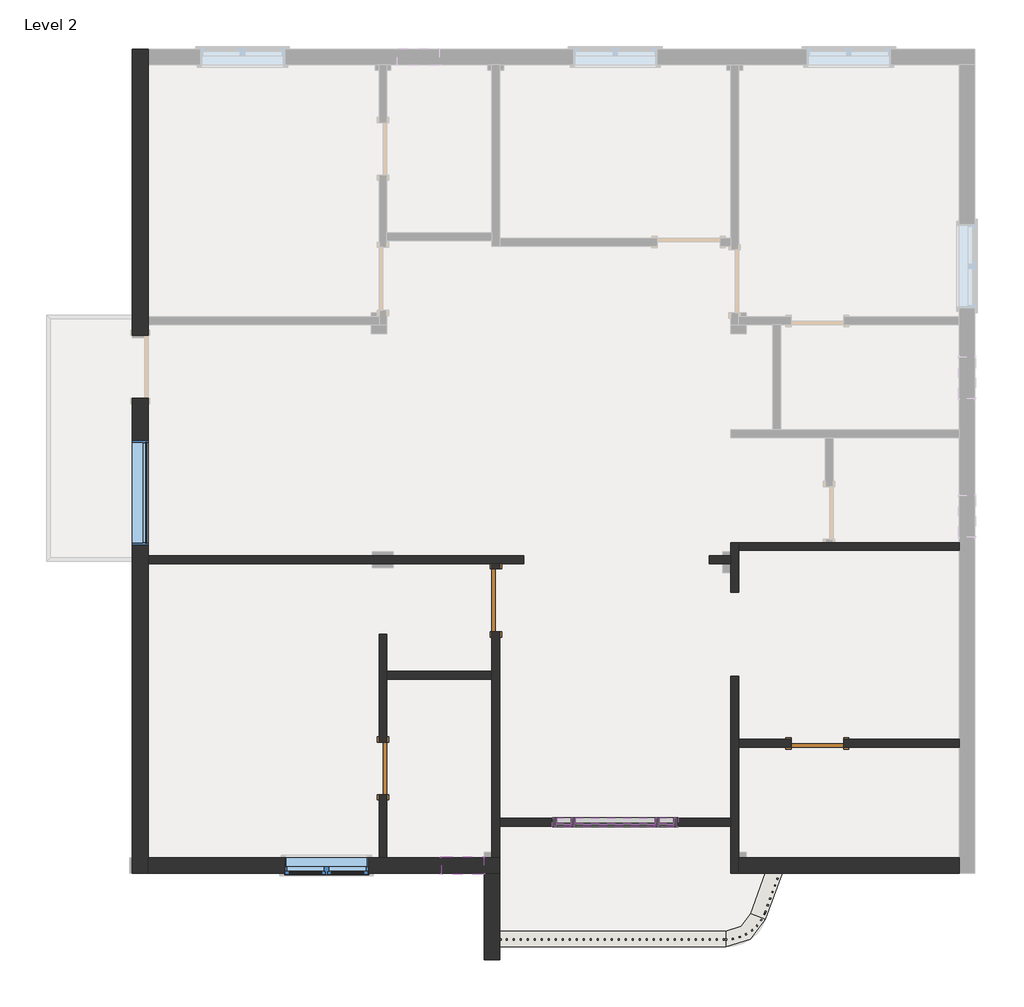
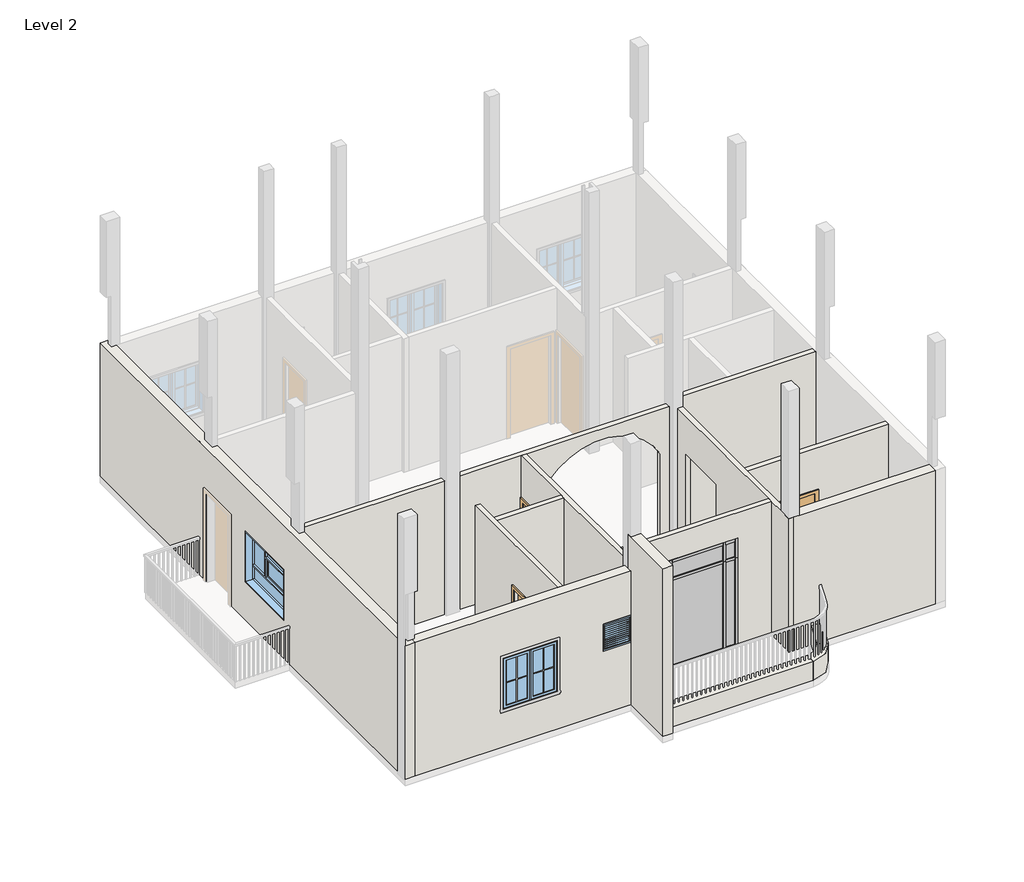
# One storey, part 1 of 4: 17 members, 15 walls, 6 plates, 3 doors, 3 windows.
"""IFC4 building model written with IfcOpenShell, lengths in millimetres."""

from ifc_helpers import new_model, si_unit, point, frame, frame_2d, origin, place, context, project, spatial, polyline, circle_curve, trimmed, segment, composite_curve, outline, extrude, faceted_brep, transform, mapped, element, save
from ifc_brep_helpers import plane_surface, revolved_surface, advanced_brep
from components import door_78caadf7, door_214872d5, door_e5f9f3c4, member_420b45ef, member_7cbddb58, member_a5966c2a, member_0585f7b2, member_d7472725, member_ffd4c858, member_15823cb3, member_3374d9b6, system_panel_glazed_ab75977c, system_panel_glazed_55699693, system_panel_glazed_94a389e0, system_panel_glazed_496eb5f8, window_awning_variable_5_x4_e7258766, window_af3140d2, window_f2d8fef0

model = new_model("IFC4")

# Units and contexts
model_context = context("Model", 3, world=origin())
ifc_project = project(units=[si_unit("LENGTHUNIT", "METRE", prefix="MILLI")], contexts=[model_context])

# Site, building, storey
site = spatial("IfcSite", under=ifc_project)
building = spatial("IfcBuilding", under=site)
storey = spatial("IfcBuildingStorey", under=building, Name="Level 2", Elevation=3200.4)

# Doors
placement = place(None, origin())
door_shape = door_78caadf7(model_context)
element("IfcDoor", 1, ObjectType="Single-Flush : 2'6\"x 7'", at=placement, inside=storey, context=model_context, shape_type="MappedRepresentation", body=[
    mapped(door_shape, transform((-11257.4178125, 3092.216018, 3200.4), x_axis=(0.0, 1.0, 0.0), y_axis=(-1.0, 0.0, 0.0), z_axis=(0.0, 0.0, 1.0))),
])
door_2_shape = door_214872d5(model_context)
element("IfcDoor", 2, ObjectType="Single-Flush : 2'6\"x 7'", at=placement, inside=storey, context=model_context, shape_type="MappedRepresentation", body=[
    mapped(door_2_shape, transform((-4951.8678125, 3454.166018, 3200.4), x_axis=(-1.0, 0.0, 0.0), y_axis=(0.0, -1.0, 0.0), z_axis=(0.0, 0.0, 1.0))),
])
door_3_shape = door_e5f9f3c4(model_context)
element("IfcDoor", 3, ObjectType="Single-Flush : 36\" x 84\"", at=placement, inside=storey, context=model_context, shape_type="MappedRepresentation", body=[
    mapped(door_3_shape, transform((-9619.1178125, 5530.616018, 3200.4), x_axis=(0.0, 1.0, 0.0), y_axis=(-1.0, 0.0, 0.0), z_axis=(0.0, 0.0, 1.0))),
])

# Members
member_shape = member_420b45ef(model_context)
element("IfcMember", 4, ObjectType="Rectangular Mullion : 2.5\" x 5\" rectangular", at=placement, inside=storey, context=model_context, shape_type="MappedRepresentation", body=[
    mapped(member_shape, transform((-8736.4678125, 2311.166018, 5791.2), x_axis=(0.0, 0.0, 1.0), y_axis=(0.0, 1.0, 0.0), z_axis=(-1.0, 0.0, 0.0))),
])
element("IfcMember", 5, ObjectType="Rectangular Mullion : 2.5\" x 5\" rectangular", at=placement, inside=storey, context=model_context, shape_type="MappedRepresentation", body=[
    mapped(member_shape, transform((-7244.2178125, 2311.166018, 5791.2), x_axis=(0.0, 0.0, 1.0), y_axis=(0.0, 1.0, 0.0), z_axis=(-1.0, 0.0, 0.0))),
])
element("IfcMember", 6, ObjectType="Rectangular Mullion : 2.5\" x 5\" rectangular", at=placement, inside=storey, context=model_context, shape_type="MappedRepresentation", body=[
    mapped(member_shape, transform((-7034.6678125, 2311.166018, 3200.4), x_axis=(0.0, 0.0, -1.0), y_axis=(0.0, 1.0, 0.0), z_axis=(1.0, 0.0, 0.0))),
])
element("IfcMember", 7, ObjectType="Rectangular Mullion : 2.5\" x 5\" rectangular", at=placement, inside=storey, context=model_context, shape_type="MappedRepresentation", body=[
    mapped(member_shape, transform((-8526.9178125, 2311.166018, 3200.4), x_axis=(0.0, 0.0, -1.0), y_axis=(0.0, 1.0, 0.0), z_axis=(1.0, 0.0, 0.0))),
])
member_2_shape = member_7cbddb58(model_context)
element("IfcMember", 8, ObjectType="Rectangular Mullion : 2.5\" x 5\" rectangular", at=placement, inside=storey, context=model_context, shape_type="MappedRepresentation", body=[
    mapped(member_2_shape, transform((-7275.9678125, 2311.166018, 3200.4), x_axis=(-1.0, 0.0, 0.0), y_axis=(0.0, 1.0, 0.0), z_axis=(0.0, 0.0, -1.0))),
])
element("IfcMember", 9, ObjectType="Rectangular Mullion : 2.5\" x 5\" rectangular", at=placement, inside=storey, context=model_context, shape_type="MappedRepresentation", body=[
    mapped(member_2_shape, transform((-8495.1678125, 2311.166018, 3200.4), x_axis=(-1.0, 0.0, 0.0), y_axis=(0.0, 1.0, 0.0), z_axis=(0.0, 0.0, -1.0))),
])
member_3_shape = member_a5966c2a(model_context)
element("IfcMember", 10, ObjectType="Rectangular Mullion : 2.5\" x 5\" rectangular", at=placement, inside=storey, context=model_context, shape_type="MappedRepresentation", body=[
    mapped(member_3_shape, transform((-7244.2178125, 2311.166018, 5334.0), x_axis=(0.0, 0.0, 1.0), y_axis=(0.0, 1.0, 0.0), z_axis=(-1.0, 0.0, 0.0))),
])
element("IfcMember", 11, ObjectType="Rectangular Mullion : 2.5\" x 5\" rectangular", at=placement, inside=storey, context=model_context, shape_type="MappedRepresentation", body=[
    mapped(member_3_shape, transform((-8736.4678125, 2311.166018, 5334.0), x_axis=(0.0, 0.0, 1.0), y_axis=(0.0, 1.0, 0.0), z_axis=(-1.0, 0.0, 0.0))),
])
member_4_shape = member_0585f7b2(model_context)
element("IfcMember", 12, ObjectType="Rectangular Mullion : 2.5\" x 5\" rectangular", at=placement, inside=storey, context=model_context, shape_type="MappedRepresentation", body=[
    mapped(member_4_shape, transform((-8463.4178125, 2311.166018, 5334.0), x_axis=(0.0, 0.0, 1.0), y_axis=(0.0, 1.0, 0.0), z_axis=(-1.0, 0.0, 0.0))),
])
member_5_shape = member_d7472725(model_context)
element("IfcMember", 13, ObjectType="Rectangular Mullion : 2.5\" x 5\" rectangular", at=placement, inside=storey, context=model_context, shape_type="MappedRepresentation", body=[
    mapped(member_5_shape, transform((-7307.7178125, 2311.166018, 3200.4), x_axis=(0.0, 0.0, -1.0), y_axis=(0.0, 1.0, 0.0), z_axis=(1.0, 0.0, 0.0))),
])
element("IfcMember", 14, ObjectType="Rectangular Mullion : 2.5\" x 5\" rectangular", at=placement, inside=storey, context=model_context, shape_type="MappedRepresentation", body=[
    mapped(member_5_shape, transform((-8463.4178125, 2311.166018, 5791.2), x_axis=(0.0, 0.0, 1.0), y_axis=(0.0, 1.0, 0.0), z_axis=(-1.0, 0.0, 0.0))),
])
member_6_shape = member_ffd4c858(model_context)
element("IfcMember", 15, ObjectType="Rectangular Mullion : 2.5\" x 5\" rectangular", at=placement, inside=storey, context=model_context, shape_type="MappedRepresentation", body=[
    mapped(member_6_shape, transform((-7275.9678125, 2311.166018, 5334.0), x_axis=(-1.0, 0.0, 0.0), y_axis=(0.0, 1.0, 0.0), z_axis=(0.0, 0.0, -1.0))),
])
element("IfcMember", 16, ObjectType="Rectangular Mullion : 2.5\" x 5\" rectangular", at=placement, inside=storey, context=model_context, shape_type="MappedRepresentation", body=[
    mapped(member_6_shape, transform((-8495.1678125, 2311.166018, 5334.0), x_axis=(-1.0, 0.0, 0.0), y_axis=(0.0, 1.0, 0.0), z_axis=(0.0, 0.0, -1.0))),
])
member_7_shape = member_15823cb3(model_context)
element("IfcMember", 17, ObjectType="Rectangular Mullion : 2.5\" x 5\" rectangular", at=placement, inside=storey, context=model_context, shape_type="MappedRepresentation", body=[
    mapped(member_7_shape, transform((-6971.1678125, 2311.166018, 5791.2), x_axis=(1.0, 0.0, 0.0), y_axis=(0.0, 1.0, 0.0), z_axis=(0.0, 0.0, 1.0))),
])
member_8_shape = member_3374d9b6(model_context)
element("IfcMember", 18, ObjectType="Rectangular Mullion : 2.5\" x 5\" rectangular", at=placement, inside=storey, context=model_context, shape_type="MappedRepresentation", body=[
    mapped(member_8_shape, transform((-8799.9678125, 2311.166018, 3200.4), x_axis=(-1.0, 0.0, 0.0), y_axis=(0.0, 1.0, 0.0), z_axis=(0.0, 0.0, -1.0))),
])
element("IfcMember", 19, ObjectType="Rectangular Mullion : 2.5\" x 5\" rectangular", at=placement, inside=storey, context=model_context, shape_type="MappedRepresentation", body=[
    mapped(member_7_shape, transform((-8799.9678125, 2311.166018, 5334.0), x_axis=(-1.0, 0.0, 0.0), y_axis=(0.0, 1.0, 0.0), z_axis=(0.0, 0.0, -1.0))),
])
element("IfcMember", 20, ObjectType="Rectangular Mullion : 2.5\" x 5\" rectangular", at=placement, inside=storey, context=model_context, shape_type="MappedRepresentation", body=[
    mapped(member_8_shape, transform((-6971.1678125, 2311.166018, 5334.0), x_axis=(1.0, 0.0, 0.0), y_axis=(0.0, 1.0, 0.0), z_axis=(0.0, 0.0, 1.0))),
])

# Plates
system_panel_glazed_shape = system_panel_glazed_ab75977c(model_context)
element("IfcPlate", 21, ObjectType="System Panel : Glazed", at=placement, inside=storey, context=model_context, shape_type="MappedRepresentation", body=[
    mapped(system_panel_glazed_shape, transform((-7139.4428125, 2311.166018, 3263.9), x_axis=(-1.0, 0.0, 0.0), y_axis=(0.0, -1.0, 0.0), z_axis=(0.0, 0.0, 1.0))),
])
element("IfcPlate", 22, ObjectType="System Panel : Glazed", at=placement, inside=storey, context=model_context, shape_type="MappedRepresentation", body=[
    mapped(system_panel_glazed_shape, transform((-8631.6928125, 2311.166018, 3263.9), x_axis=(-1.0, 0.0, 0.0), y_axis=(0.0, -1.0, 0.0), z_axis=(0.0, 0.0, 1.0))),
])
system_panel_glazed_2_shape = system_panel_glazed_55699693(model_context)
element("IfcPlate", 23, ObjectType="System Panel : Glazed", at=placement, inside=storey, context=model_context, shape_type="MappedRepresentation", body=[
    mapped(system_panel_glazed_2_shape, transform((-7885.5678125, 2311.166018, 3263.9), x_axis=(-1.0, 0.0, 0.0), y_axis=(0.0, -1.0, 0.0), z_axis=(0.0, 0.0, 1.0))),
])
system_panel_glazed_3_shape = system_panel_glazed_94a389e0(model_context)
element("IfcPlate", 24, ObjectType="System Panel : Glazed", at=placement, inside=storey, context=model_context, shape_type="MappedRepresentation", body=[
    mapped(system_panel_glazed_3_shape, transform((-7139.4428125, 2311.166018, 5365.75), x_axis=(-1.0, 0.0, 0.0), y_axis=(0.0, -1.0, 0.0), z_axis=(0.0, 0.0, 1.0))),
])
element("IfcPlate", 25, ObjectType="System Panel : Glazed", at=placement, inside=storey, context=model_context, shape_type="MappedRepresentation", body=[
    mapped(system_panel_glazed_3_shape, transform((-8631.6928125, 2311.166018, 5365.75), x_axis=(-1.0, 0.0, 0.0), y_axis=(0.0, -1.0, 0.0), z_axis=(0.0, 0.0, 1.0))),
])
system_panel_glazed_4_shape = system_panel_glazed_496eb5f8(model_context)
element("IfcPlate", 26, ObjectType="System Panel : Glazed", at=placement, inside=storey, context=model_context, shape_type="MappedRepresentation", body=[
    mapped(system_panel_glazed_4_shape, transform((-7885.5678125, 2311.166018, 5365.75), x_axis=(-1.0, 0.0, 0.0), y_axis=(0.0, -1.0, 0.0), z_axis=(0.0, 0.0, 1.0))),
])

# Walls
element("IfcWall", 27, ObjectType="4.5\" wall", at=placement, inside=storey, context=model_context, shape_type="AdvancedBrep", body=[
    advanced_brep(
    [(-14667.3678125, 6064.016018, 3200.4), (-11409.8178125, 6064.016018, 3200.4), (-11105.0178125, 6064.016018, 3200.4), (-9676.2678125, 6064.016018, 3200.4), (-9561.9678125, 6064.016018, 3200.4), (-9216.6666467, 6064.016018, 3200.4), (-9216.6666467, 6064.016018, 5334.0), (-6524.2666467, 6064.016018, 5334.0), (-6524.2666467, 6064.016018, 3200.4), (-6323.4678125, 6064.016018, 3200.4), (-6209.1678125, 6064.016018, 3200.4), (-6209.1678125, 6064.016018, 6400.8), (-6323.4678125, 6064.016018, 6400.8), (-9561.9678125, 6064.016018, 6400.8), (-9676.2678125, 6064.016018, 6400.8), (-11105.0178125, 6064.016018, 6400.8), (-11409.8178125, 6064.016018, 6400.8), (-14667.3678125, 6064.016018, 6400.8), (-14667.3678125, 6178.316018, 3200.4), (-14667.3678125, 6178.316018, 6400.8), (-11409.8178125, 6178.316018, 6400.8), (-11105.0178125, 6178.316018, 6400.8), (-6323.4678125, 6178.316018, 6400.8), (-6209.1678125, 6178.316018, 6400.8), (-6209.1678125, 6178.316018, 3200.4), (-6323.4678125, 6178.316018, 3200.4), (-6524.2666467, 6178.316018, 3200.4), (-6524.2666467, 6178.316018, 5334.0), (-9216.6666467, 6178.316018, 5334.0), (-9216.6666467, 6178.316018, 3200.4), (-11105.0178125, 6178.316018, 3200.4), (-11409.8178125, 6178.316018, 3200.4)],
    [
        (0, 1),
        (1, 2),
        (2, 3),
        (3, 4),
        (4, 5),
        (5, 6),
        (6, 7, circle_curve(frame((-7870.4666467, 6064.016018, 4634.1183788), z_axis=(0.0, 1.0, 0.0), x_axis=(-1.0, 0.0, 0.0)), 1517.2635644)),
        (7, 8),
        (8, 9),
        (9, 10),
        (10, 11),
        (11, 12),
        (12, 13),
        (13, 14),
        (14, 15),
        (15, 16),
        (16, 17),
        (17, 0),
        (18, 19),
        (19, 20),
        (20, 21),
        (21, 22),
        (22, 23),
        (23, 24),
        (24, 25),
        (25, 26),
        (26, 27),
        (27, 28, circle_curve(frame((-7870.4666467, 6178.316018, 4634.1183788), z_axis=(0.0, -1.0, 0.0), x_axis=(-1.0, 0.0, 0.0)), 1517.2635644)),
        (28, 29),
        (29, 30),
        (30, 31),
        (31, 18),
        (17, 19),
        (18, 0),
        (10, 24),
        (23, 11),
        (29, 5),
        (28, 6),
        (27, 7),
        (26, 8),
    ],
    [
        plane_surface(frame((-14781.6678125, 6064.016018, 3200.4), z_axis=(0.0, -1.0, 0.0), x_axis=(1.0, 0.0, 0.0))),
        plane_surface(frame((-14781.6678125, 6178.316018, 3200.4), z_axis=(0.0, 1.0, 0.0), x_axis=(-1.0, 0.0, 0.0))),
        plane_surface(frame((-14667.3678125, 13531.616018, 3200.4), z_axis=(-1.0, 0.0, 0.0), x_axis=(0.0, 1.0, 0.0))),
        plane_surface(frame((-6209.1678125, 6010.7399841, 3200.4), z_axis=(1.0, 0.0, 0.0), x_axis=(0.0, -1.0, 0.0))),
        plane_surface(frame((-14781.6678125, 6064.016018, 3200.4), z_axis=(0.0, 0.0, -1.0), x_axis=(0.0, 1.0, 0.0))),
        plane_surface(frame((-6152.0178125, 6064.016018, 6400.8), z_axis=(0.0, 0.0, 1.0), x_axis=(0.0, 1.0, 0.0))),
        plane_surface(frame((-9216.6666467, 6064.016018, 3200.4), z_axis=(1.0, 0.0, 0.0), x_axis=(0.0, 1.0, 0.0))),
        revolved_surface(polyline([(-9387.730211099999, 6178.316018, 4634.1183788), (-9387.730211099999, 6064.016018, 4634.1183788)]), (-7870.4666467, 6178.316018, 4634.1183788), (0.0, 1.0, 0.0)),
        plane_surface(frame((-6524.2666467, 6064.016018, 5334.0), z_axis=(-1.0, 0.0, 0.0), x_axis=(0.0, 1.0, 0.0))),
        plane_surface(frame((-6524.2666467, 6064.016018, 3200.4), z_axis=(0.0, 0.0, -1.0), x_axis=(0.0, 1.0, 0.0))),
    ],
    [
        (0, [[1, 2, 3, 4, 5, 6, 7, 8, 9, 10, 11, 12, 13, 14, 15, 16, 17, 18]]),
        (1, [[19, 20, 21, 22, 23, 24, 25, 26, 27, 28, 29, 30, 31, 32]]),
        (2, [[-18, 33, -19, 34]]),
        (3, [[-11, 35, -24, 36]]),
        (4, [[-5, -4, -3, -2, -1, -34, -32, -31, -30, 37]]),
        (5, [[-17, -16, -15, -14, -13, -12, -36, -23, -22, -21, -20, -33]]),
        (6, [[-6, -37, -29, 38]]),
        (7, [[-7, -38, -28, 39]]),
        (8, [[-8, -39, -27, 40]]),
        (9, [[-10, -9, -40, -26, -25, -35]]),
    ],
),
])
element("IfcWall", 28, ObjectType="4.5\" wall", at=placement, inside=storey, context=model_context, shape_type="Brep", body=[
    faceted_brep([(-11314.5678125, 5035.316018, 3200.4), (-11314.5678125, 3473.216018, 3200.4), (-11314.5678125, 3473.216018, 5334.0), (-11314.5678125, 2711.216018, 5334.0), (-11314.5678125, 2711.216018, 3200.4), (-11314.5678125, 1796.816018, 3200.4), (-11314.5678125, 1796.816018, 6400.8), (-11314.5678125, 5035.316018, 6400.8), (-11200.2678125, 3473.216018, 5334.0), (-11200.2678125, 3473.216018, 3200.4), (-11200.2678125, 4387.616018, 3200.4), (-11200.2678125, 4501.916018, 3200.4), (-11200.2678125, 5035.316018, 3200.4), (-11200.2678125, 5035.316018, 6400.8), (-11200.2678125, 4501.916018, 6400.8), (-11200.2678125, 4387.616018, 6400.8), (-11200.2678125, 1796.816018, 6400.8), (-11200.2678125, 1796.816018, 3200.4), (-11200.2678125, 2711.216018, 3200.4), (-11200.2678125, 2711.216018, 5334.0)], [[[0, 1, 2, 3, 4, 5, 6, 7]], [[8, 9, 10, 11, 12, 13, 14, 15, 16, 17, 18, 19]], [[18, 17, 5, 4]], [[12, 11, 10, 9, 1, 0]], [[7, 6, 16, 15, 14, 13]], [[0, 7, 13, 12]], [[6, 5, 17, 16]], [[2, 1, 9, 8]], [[3, 2, 8, 19]], [[4, 3, 19, 18]]]),
])
element("IfcWall", 29, ObjectType="4.5\" wall", at=placement, inside=storey, context=model_context, shape_type="Brep", body=[
    faceted_brep([(-9561.9678125, 5987.816018, 5334.0), (-9561.9678125, 5987.816018, 3200.4), (-9561.9678125, 6064.016018, 3200.4), (-9561.9678125, 6064.016018, 6400.8), (-9561.9678125, 2368.316018, 6400.8), (-9561.9678125, 2254.016018, 6400.8), (-9561.9678125, 1873.016018, 6400.8), (-9561.9678125, 1796.816018, 6400.8), (-9561.9678125, 1796.816018, 3200.4), (-9561.9678125, 2254.016018, 3200.4), (-9561.9678125, 2368.316018, 3200.4), (-9561.9678125, 5073.416018, 3200.4), (-9561.9678125, 5073.416018, 5334.0), (-9676.2678125, 6064.016018, 3200.4), (-9676.2678125, 5987.816018, 3200.4), (-9676.2678125, 5987.816018, 5334.0), (-9676.2678125, 5073.416018, 5334.0), (-9676.2678125, 5073.416018, 3200.4), (-9676.2678125, 4501.916018, 3200.4), (-9676.2678125, 4387.616018, 3200.4), (-9676.2678125, 1873.016018, 3200.4), (-9676.2678125, 1796.816018, 3200.4), (-9676.2678125, 1796.816018, 6400.8), (-9676.2678125, 1873.016018, 6400.8), (-9676.2678125, 4387.616018, 6400.8), (-9676.2678125, 4501.916018, 6400.8), (-9676.2678125, 6064.016018, 6400.8)], [[[0, 1, 2, 3, 4, 5, 6, 7, 8, 9, 10, 11, 12]], [[13, 14, 15, 16, 17, 18, 19, 20, 21, 22, 23, 24, 25, 26]], [[2, 1, 14, 13]], [[11, 10, 9, 8, 21, 20, 19, 18, 17]], [[7, 6, 5, 4, 3, 26, 25, 24, 23, 22]], [[8, 7, 22, 21]], [[15, 14, 1, 0]], [[16, 15, 0, 12]], [[17, 16, 12, 11]], [[3, 2, 13, 26]]]),
])
element("IfcWall", 30, ObjectType="4.5\" wall", at=placement, inside=storey, context=model_context, shape_type="SweptSolid", body=[
    extrude(outline(polyline([(-9676.2678125, 4387.616018), (-11200.2678125, 4387.616018), (-11200.2678125, 4501.916018), (-9676.2678125, 4501.916018), (-9676.2678125, 4387.616018)])), frame((0.0, 0.0, 3200.4), z_axis=(0.0, 0.0, 1.0), x_axis=(1.0, 0.0, 0.0)), (0.0, 0.0, 1.0), 3200.4),
])
element("IfcWall", 31, ObjectType="4.5\" wall", at=placement, inside=storey, context=model_context, shape_type="Brep", body=[
    faceted_brep([(-6094.8678125, 6368.816018, 3200.4), (-6094.8678125, 6368.816018, 6400.8), (-6094.8678125, 6254.516018, 6400.8), (-6094.8678125, 6235.466018, 6400.8), (-6094.8678125, 5930.666018, 6400.8), (-6094.8678125, 3511.316018, 6400.8), (-6094.8678125, 3397.016018, 6400.8), (-6094.8678125, 1873.016018, 6400.8), (-6094.8678125, 1796.816018, 6400.8), (-6094.8678125, 1568.216018, 6400.8), (-6094.8678125, 1568.216018, 3200.4), (-6094.8678125, 1796.816018, 3200.4), (-6094.8678125, 1873.016018, 3200.4), (-6094.8678125, 3397.016018, 3200.4), (-6094.8678125, 3511.316018, 3200.4), (-6094.8678125, 4425.716018, 3200.4), (-6094.8678125, 4425.716018, 5486.4), (-6094.8678125, 5644.916018, 5486.4), (-6094.8678125, 5644.916018, 3200.4), (-6094.8678125, 6254.516018, 3200.4), (-6209.1678125, 6368.816018, 6400.8), (-6209.1678125, 6368.816018, 3200.4), (-6209.1678125, 6235.466018, 3200.4), (-6209.1678125, 6178.316018, 3200.4), (-6209.1678125, 6064.016018, 3200.4), (-6209.1678125, 5930.666018, 3200.4), (-6209.1678125, 5644.916018, 3200.4), (-6209.1678125, 5644.916018, 5486.4), (-6209.1678125, 4425.716018, 5486.4), (-6209.1678125, 4425.716018, 3200.4), (-6209.1678125, 2368.316018, 3200.4), (-6209.1678125, 2254.016018, 3200.4), (-6209.1678125, 1568.216018, 3200.4), (-6209.1678125, 1568.216018, 6400.8), (-6209.1678125, 1873.016018, 6400.8), (-6209.1678125, 2254.016018, 6400.8), (-6209.1678125, 2368.316018, 6400.8), (-6209.1678125, 5930.666018, 6400.8), (-6209.1678125, 6064.016018, 6400.8), (-6209.1678125, 6178.316018, 6400.8), (-6209.1678125, 6235.466018, 6400.8)], [[[0, 1, 2, 3, 4, 5, 6, 7, 8, 9, 10, 11, 12, 13, 14, 15, 16, 17, 18, 19]], [[20, 21, 22, 23, 24, 25, 26, 27, 28, 29, 30, 31, 32, 33, 34, 35, 36, 37, 38, 39, 40]], [[21, 0, 19, 18, 26, 25, 24, 23, 22]], [[10, 32, 31, 30, 29, 15, 14, 13, 12, 11]], [[9, 8, 7, 6, 5, 4, 3, 2, 1, 20, 40, 39, 38, 37, 36, 35, 34, 33]], [[1, 0, 21, 20]], [[10, 9, 33, 32]], [[16, 28, 27, 17]], [[28, 16, 15, 29]], [[17, 27, 26, 18]]]),
])
element("IfcWall", 32, ObjectType="4.5\" wall", at=placement, inside=storey, context=model_context, shape_type="Brep", body=[
    faceted_brep([(-2894.4678125, 6368.816018, 3200.4), (-4723.2678125, 6368.816018, 3200.4), (-4837.5678125, 6368.816018, 3200.4), (-6094.8678125, 6368.816018, 3200.4), (-6094.8678125, 6368.816018, 6400.8), (-4837.5678125, 6368.816018, 6400.8), (-4723.2678125, 6368.816018, 6400.8), (-2894.4678125, 6368.816018, 6400.8), (-2894.4678125, 6254.516018, 3200.4), (-2894.4678125, 6254.516018, 6400.8), (-6094.8678125, 6254.516018, 6400.8), (-6094.8678125, 6254.516018, 3200.4)], [[[0, 1, 2, 3, 4, 5, 6, 7]], [[8, 9, 10, 11]], [[3, 2, 1, 0, 8, 11]], [[7, 6, 5, 4, 10, 9]], [[0, 7, 9, 8]], [[4, 3, 11, 10]]]),
])
element("IfcWall", 33, ObjectType="4.5\" wall", at=placement, inside=storey, context=model_context, shape_type="SweptSolid", body=[
    extrude(outline(polyline([(3200.4, -6094.8678125), (3200.4, -5332.8678125), (5334.0, -5332.8678125), (5334.0, -4570.8678125), (3200.4, -4570.8678125), (3200.4, -2894.4678125), (6400.8, -2894.4678125), (6400.8, -6094.8678125), (3200.4, -6094.8678125)])), frame((0.0, 3397.016018, 0.0), z_axis=(0.0, 1.0, 0.0), x_axis=(0.0, 0.0, 1.0)), (0.0, 0.0, 1.0), 114.3),
])
element("IfcWall", 34, ObjectType="4.5\" wall", at=placement, inside=storey, context=model_context, shape_type="SweptSolid", body=[
    extrude(outline(polyline([(6400.8, -6209.1678125), (6400.8, -9561.9678125), (3200.4, -9561.9678125), (3200.4, -8799.9678125), (5791.2, -8799.9678125), (5791.2, -6971.1678125), (3200.4, -6971.1678125), (3200.4, -6209.1678125), (6400.8, -6209.1678125)])), frame((0.0, 2254.016018, 0.0), z_axis=(0.0, 1.0, 0.0), x_axis=(0.0, 0.0, 1.0)), (0.0, 0.0, 1.0), 114.3),
])
element("IfcWall", 35, ObjectType="9\" wall", at=placement, inside=storey, context=model_context, shape_type="Brep", body=[
    faceted_brep([(-14895.9678125, 13531.616018, 3200.4), (-14895.9678125, 9645.416018, 3200.4), (-14895.9678125, 9378.716018, 3200.4), (-14895.9678125, 9378.716018, 5334.0), (-14895.9678125, 9340.616018, 5334.0), (-14895.9678125, 8464.316018, 5334.0), (-14895.9678125, 8464.316018, 3200.4), (-14895.9678125, 6235.466018, 3200.4), (-14895.9678125, 5930.666018, 3200.4), (-14895.9678125, 1796.816018, 3200.4), (-14895.9678125, 1568.216018, 3200.4), (-14895.9678125, 1568.216018, 6400.8), (-14895.9678125, 13531.616018, 6400.8), (-14895.9678125, 6330.716018, 5334.0), (-14895.9678125, 6330.716018, 4114.8), (-14895.9678125, 7854.716018, 4114.8), (-14895.9678125, 7854.716018, 5334.0), (-14667.3678125, 9378.716018, 5334.0), (-14667.3678125, 9378.716018, 3200.4), (-14667.3678125, 9531.116018, 3200.4), (-14667.3678125, 9645.416018, 3200.4), (-14667.3678125, 13303.016018, 3200.4), (-14667.3678125, 13531.616018, 3200.4), (-14667.3678125, 13531.616018, 6400.8), (-14667.3678125, 13417.316018, 6400.8), (-14667.3678125, 13303.016018, 6400.8), (-14667.3678125, 9645.416018, 6400.8), (-14667.3678125, 9531.116018, 6400.8), (-14667.3678125, 9340.616018, 6400.8), (-14667.3678125, 6235.466018, 6400.8), (-14667.3678125, 6178.316018, 6400.8), (-14667.3678125, 6064.016018, 6400.8), (-14667.3678125, 5930.666018, 6400.8), (-14667.3678125, 1796.816018, 6400.8), (-14667.3678125, 1568.216018, 6400.8), (-14667.3678125, 1568.216018, 3200.4), (-14667.3678125, 1796.816018, 3200.4), (-14667.3678125, 5930.666018, 3200.4), (-14667.3678125, 6064.016018, 3200.4), (-14667.3678125, 6178.316018, 3200.4), (-14667.3678125, 6235.466018, 3200.4), (-14667.3678125, 8464.316018, 3200.4), (-14667.3678125, 8464.316018, 5334.0), (-14667.3678125, 9340.616018, 5334.0), (-14667.3678125, 6330.716018, 5334.0), (-14667.3678125, 7854.716018, 5334.0), (-14667.3678125, 7854.716018, 4114.8), (-14667.3678125, 6330.716018, 4114.8)], [[[0, 1, 2, 3, 4, 5, 6, 7, 8, 9, 10, 11, 12], [13, 14, 15, 16]], [[17, 18, 19, 20, 21, 22, 23, 24, 25, 26, 27, 28, 29, 30, 31, 32, 33, 34, 35, 36, 37, 38, 39, 40, 41, 42, 43], [44, 45, 46, 47]], [[22, 21, 20, 19, 18, 2, 1, 0]], [[41, 40, 39, 38, 37, 36, 35, 10, 9, 8, 7, 6]], [[12, 11, 34, 33, 32, 31, 30, 29, 28, 27, 26, 25, 24, 23]], [[0, 12, 23, 22]], [[11, 10, 35, 34]], [[14, 13, 44, 47]], [[15, 14, 47, 46]], [[16, 15, 46, 45]], [[13, 16, 45, 44]], [[3, 2, 18, 17]], [[5, 4, 3, 17, 43, 42]], [[6, 5, 42, 41]]]),
])
element("IfcWall", 36, ObjectType="9\" wall", at=placement, inside=storey, context=model_context, shape_type="Brep", body=[
    faceted_brep([(-14667.3678125, 1568.216018, 3200.4), (-9790.5678125, 1568.216018, 3200.4), (-9561.9678125, 1568.216018, 3200.4), (-9561.9678125, 1568.216018, 6400.8), (-9790.5678125, 1568.216018, 6400.8), (-14667.3678125, 1568.216018, 6400.8), (-9796.9178125, 1568.216018, 5334.0), (-9796.9178125, 1568.216018, 4724.4), (-10406.5178125, 1568.216018, 4724.4), (-10406.5178125, 1568.216018, 5334.0), (-12686.1678125, 1568.216018, 5334.0), (-11466.9678125, 1568.216018, 5334.0), (-11466.9678125, 1568.216018, 4114.8), (-12686.1678125, 1568.216018, 4114.8), (-14667.3678125, 1796.816018, 3200.4), (-14667.3678125, 1796.816018, 6400.8), (-14629.2678125, 1796.816018, 6400.8), (-11314.5678125, 1796.816018, 6400.8), (-11200.2678125, 1796.816018, 6400.8), (-9790.5678125, 1796.816018, 6400.8), (-9676.2678125, 1796.816018, 6400.8), (-9561.9678125, 1796.816018, 6400.8), (-9561.9678125, 1796.816018, 3200.4), (-9676.2678125, 1796.816018, 3200.4), (-9790.5678125, 1796.816018, 3200.4), (-11200.2678125, 1796.816018, 3200.4), (-11314.5678125, 1796.816018, 3200.4), (-9796.9178125, 1796.816018, 5334.0), (-10406.5178125, 1796.816018, 5334.0), (-10406.5178125, 1796.816018, 4724.4), (-9796.9178125, 1796.816018, 4724.4), (-12686.1678125, 1796.816018, 5334.0), (-12686.1678125, 1796.816018, 4114.8), (-11466.9678125, 1796.816018, 4114.8), (-11466.9678125, 1796.816018, 5334.0), (-9561.9678125, 1682.516018, 6400.8)], [[[0, 1, 2, 3, 4, 5], [6, 7, 8, 9], [10, 11, 12, 13]], [[14, 15, 16, 17, 18, 19, 20, 21, 22, 23, 24, 25, 26], [27, 28, 29, 30], [31, 32, 33, 34]], [[2, 1, 0, 14, 26, 25, 24, 23, 22]], [[5, 4, 3, 35, 21, 20, 19, 18, 17, 16, 15]], [[0, 5, 15, 14]], [[3, 2, 22, 21, 35]], [[7, 6, 27, 30]], [[8, 7, 30, 29]], [[9, 8, 29, 28]], [[6, 9, 28, 27]], [[32, 31, 10, 13]], [[33, 32, 13, 12]], [[34, 33, 12, 11]], [[31, 34, 11, 10]]]),
])
element("IfcWall", 37, ObjectType="9\" wall", at=placement, inside=storey, context=model_context, shape_type="SweptSolid", body=[
    extrude(outline(polyline([(-6278.443289, 501.416018), (-9561.9678125, 501.416018), (-9561.9678125, 730.016018), (-6278.443289, 730.016018), (-6278.443289, 501.416018)])), frame((0.0, 0.0, 3200.4), z_axis=(0.0, 0.0, 1.0), x_axis=(1.0, 0.0, 0.0)), (0.0, 0.0, 1.0), 457.2),
])
element("IfcWall", 38, ObjectType="9\" wall", at=placement, inside=storey, context=model_context, shape_type="Brep", body=[
    faceted_brep([(-9561.9678125, 310.916018, 3200.4), (-9561.9678125, 501.416018, 3200.4), (-9561.9678125, 730.016018, 3200.4), (-9561.9678125, 1568.216018, 3200.4), (-9561.9678125, 1568.216018, 6400.8), (-9561.9678125, 1682.516018, 6400.8), (-9561.9678125, 1682.516018, 7218.0977729), (-9561.9678125, 1568.216018, 7218.0977729), (-9561.9678125, 310.916018, 7218.0977729), (-9790.5678125, 310.916018, 3200.4), (-9790.5678125, 310.916018, 7218.0977729), (-9790.5678125, 1568.216018, 7218.0977729), (-9790.5678125, 1682.516018, 7218.0977729), (-9790.5678125, 1682.516018, 6400.8), (-9790.5678125, 1568.216018, 6400.8), (-9790.5678125, 1568.216018, 3200.4)], [[[0, 1, 2, 3, 4, 5, 6, 7, 8]], [[9, 10, 11, 12, 13, 14, 15]], [[3, 2, 1, 0, 9, 15]], [[8, 7, 6, 12, 11, 10]], [[0, 8, 10, 9]], [[13, 5, 4, 14]], [[4, 3, 15, 14]], [[6, 5, 13, 12]]]),
])
element("IfcWall", 39, ObjectType="9\" wall", at=placement, inside=storey, context=model_context, shape_type="Brep", body=[
    faceted_brep([(-6094.8678125, 1568.216018, 3200.4), (-5706.5843666, 1568.216018, 3200.4), (-5463.3133278, 1568.216018, 3200.4), (-2894.4678125, 1568.216018, 3200.4), (-2894.4678125, 1568.216018, 6400.8), (-5980.5678125, 1568.216018, 6400.8), (-6094.8678125, 1568.216018, 6400.8), (-6094.8678125, 1796.816018, 3200.4), (-6094.8678125, 1796.816018, 6400.8), (-5980.5678125, 1796.816018, 6400.8), (-2894.4678125, 1796.816018, 6400.8), (-2894.4678125, 1796.816018, 3200.4), (-5980.5678125, 1796.816018, 3200.4), (-2894.4678125, 1682.516018, 6400.8)], [[[0, 1, 2, 3, 4, 5, 6]], [[7, 8, 9, 10, 11, 12]], [[3, 2, 1, 0, 7, 12, 11]], [[6, 5, 4, 13, 10, 9, 8]], [[4, 3, 11, 10, 13]], [[0, 6, 8, 7]]]),
])
element("IfcWall", 40, ObjectType="9\" wall", at=placement, inside=storey, context=model_context, shape_type="SweptSolid", body=[
    extrude(outline(polyline([(-5463.3133278, 1568.216018), (-5705.6066674, 902.5205386), (-5920.4204005, 980.7063434), (-5706.5843666, 1568.216018), (-5463.3133278, 1568.216018)])), frame((0.0, 0.0, 3200.4), z_axis=(0.0, 0.0, 1.0), x_axis=(1.0, 0.0, 0.0)), (0.0, 0.0, 1.0), 457.2),
])
element("IfcWall", 41, ObjectType="9\" wall", at=placement, inside=storey, context=model_context, shape_type="SweptSolid", body=[
    extrude(outline(composite_curve([segment(polyline([(-5920.4204005, 980.7063434), (-5705.6066674, 902.5205386)]), True, "CONTINUOUS"), segment(trimmed(circle_curve(frame_2d((-6278.443289, 1111.016018)), 609.6), [point((-5705.6066674, 902.5205386))], [point((-6278.443289, 501.416018))], False, "CARTESIAN"), True, "CONTINUOUS"), segment(polyline([(-6278.443289, 501.416018), (-6278.443289, 730.016018)]), True, "CONTINUOUS"), segment(trimmed(circle_curve(frame_2d((-6278.443289, 1111.016018)), 381.0), [point((-6278.443289, 730.016018))], [point((-5920.4204005, 980.7063434))], True, "CARTESIAN"), True, "CONTINUOUS")], self_intersect=False)), frame((0.0, 0.0, 3200.4), z_axis=(0.0, 0.0, 1.0), x_axis=(1.0, 0.0, 0.0)), (0.0, 0.0, 1.0), 457.2),
])

# Windows
window_awning_variable_5_x4_shape = window_awning_variable_5_x4_e7258766(model_context)
element("IfcWindow", 42, ObjectType="Window-Awning-Variable : 5'x4'", at=placement, inside=storey, context=model_context, shape_type="MappedRepresentation", body=[
    mapped(window_awning_variable_5_x4_shape, transform((-14781.6678125, 7092.716018, 3200.4), x_axis=(0.0, -1.0, 0.0), y_axis=(1.0, 0.0, 0.0), z_axis=(0.0, 0.0, 1.0))),
])
window_shape = window_af3140d2(model_context)
element("IfcWindow", 43, ObjectType="Window-Casement-Double : 48\" x 48\"", at=placement, inside=storey, context=model_context, shape_type="MappedRepresentation", body=[
    mapped(window_shape, transform((-12076.5678125, 1682.516018, 3200.4), x_axis=(-1.0, 0.0, 0.0), y_axis=(0.0, -1.0, 0.0), z_axis=(0.0, 0.0, 1.0))),
])
window_2_shape = window_f2d8fef0(model_context)
element("IfcWindow", 44, ObjectType="Window-Louvers : 24\" x 24\"", at=placement, inside=storey, context=model_context, shape_type="MappedRepresentation", body=[
    mapped(window_2_shape, transform((-10101.7178125, 1676.166018, 3810.0), x_axis=(-1.0, 0.0, 0.0), y_axis=(0.0, -1.0, 0.0), z_axis=(0.0, 0.0, 1.0))),
])

save(model, "model.ifc")

# Revit data of these elements
# Type "Single-Flush : 2'6\"x 7'"
#   Type Mark = "8"
#   Construction Type Id = "MDOOR"
#   Assembly Code = "C1020"
#   Analytic Construction = "Metal"
#   Thickness = 0' - 2"
#   Heat Transfer Coefficient (U) = 0.651978 BTU/(h·ft²·°F)
#   Height = 7' - 0"
#   Trim Projection Ext = 0' - 1"
#   Trim Projection Int = 0' - 1"
#   Trim Width = 0' - 3"
#   Width = 2' - 6"
#   Define Thermal Properties by = 1
#   Door Material = Door - Panel
#   Frame Material = Door - Frame
#   Visual Light Transmittance = 0
#   Solar Heat Gain Coefficient = 0
#   Function = (empty or 0)
#   Wall Closure = (empty or 0)
# Type "Single-Flush : 36\" x 84\""
#   Type Mark = "1"
#   Construction Type Id = "MDOOR"
#   Assembly Code = "C1020"
#   Analytic Construction = "Metal"
#   Thickness = 0' - 2"
#   Heat Transfer Coefficient (U) = 0.651978 BTU/(h·ft²·°F)
#   Height = 7' - 0"
#   Trim Projection Ext = 0' - 1"
#   Trim Projection Int = 0' - 1"
#   Trim Width = 0' - 3"
#   Width = 3' - 0"
#   Define Thermal Properties by = 1
#   Define Thermal Properties by = 1
#   Door Material = Door - Panel
#   Frame Material = Door - Frame
#   Visual Light Transmittance = 0
#   Solar Heat Gain Coefficient = 0
#   Function = (empty or 0)
#   Wall Closure = (empty or 0)
# Type "Rectangular Mullion : 2.5\" x 5\" rectangular"
#   built-in parameter 1007304 = 0.416667 (stored number, unit not read)
#   built-in parameter 1007301 = 0.104167 (stored number, unit not read)
#   built-in parameter 1007300 = 0.104167 (stored number, unit not read)
# Type "System Panel : Glazed"
#   Construction Type Id = "GSP4R"
#   Analytic Construction = "1/8 in Pilkington single glazing"
#   Visual Light Transmittance = 0.9
#   Solar Heat Gain Coefficient = 0.86
#   Heat Transfer Coefficient (U) = 1.18115 BTU/(h·ft²·°F)
#   Define Thermal Properties by = 1
# Type "4.5\" wall"
#   Assembly Code = "B2010"
#   Layers, outside or top first: 0' - 4 1/2" "Gypsum Wall Board" (function 1)
# Type "9\" wall"
#   Assembly Code = "B2010"
#   Layers, outside or top first: 0' - 9" "Gypsum Wall Board" (function 1)
# Type "Window-Awning-Variable : 5'x4'"
#   Type Mark = "23"
#   Fire Rating = "0.5h"
#   Assembly Code = "B2020100"
#   Analytic Construction = "Double glazing - domestic"
#   Window Inset [instance default] = 0' - 0 5/8"
#   Wall Thickness [instance default] = 0' - 6"
#   Visual Light Transmittance = 0.81
#   Transom Height Ratio = 0.3
#   Transom Height = 1' - 2.4"
#   Thermal Resistance (R) = 1.8146 (h·ft²·°F)/BTU
#   Solar Heat Gain Coefficient = 0.76
#   Rough Width = 5' - 0 1/2"
#   Rough Height = 4' - 0 1/2"
#   Opening Window Width = 3' - 4"
#   Opening Window Height = 1' - 7.2"
#   Heat Transfer Coefficient (U) = 0.5511 BTU/(h·ft²·°F)
#   Height = 4' - 0"
#   Frame Gap 3 [instance default] = 0' - 1 83/128"
#   Frame Gap 2 [instance default] = 0' - 0 5/8"
#   Frame Gap 1 = 0' - 1 51/128"
#   Fixed Window Width = 1' - 8"
#   Default Sill Height = 3' - 0"
#   Width = 5' - 0"
#   Frame Material = Metal - Aluminum
#   Glass Panel Material = Glass
#   Wall Closure = (empty or 0)
# Type "Window-Casement-Double : 48\" x 48\""
#   Type Mark = "16"
#   Fire Rating = "0.5h"
#   Assembly Code = "B2020100"
#   Analytic Construction = "Double glazing - domestic"
#   Frame Extension [instance default] = 0' - 0 1/4"
#   Window Inset [instance default] = 0' - 0"
#   Wall Thickness [instance default] = 0' - 6"
#   Interior Wall Closure [instance default] = 0' - 2 1/4"
#   Half Width = 2' - 0"
#   Visual Light Transmittance = 0.81
#   Thermal Resistance (R) = 1.8146 (h·ft²·°F)/BTU
#   Solar Heat Gain Coefficient = 0.76
#   Rough Width = 4' - 0 1/2"
#   Rough Height = 4' - 0 1/2"
#   Height = 4' - 0"
#   Heat Transfer Coefficient (U) = 0.5511 BTU/(h·ft²·°F)
#   Exterior Wall Closure [instance default] = 0' - 1 1/4"
#   Extension Jamb [instance default] = 0' - 2 1/4"
#   Default Sill Height = 3' - 0"
#   Width = 4' - 0"
#   Define Thermal Properties by = 0
#   Muntin Visibility = yes
#   Interior Trim Visibility [instance default] = yes
#   Exterior Trim Visibility [instance default] = yes
#   Extension Jamb Visibility [instance default] = yes
#   Interior Trim Material = Wood - Stained
#   Muntin Pattern = Muntin Pattern_2x2 : Muntin Pattern_2x2
#   Interior Trim = Trim-Window-Interior-Flat : Picture Frame
#   Interior Frame Material = Wood - Stained
#   Glass Panel Material = Glass
#   Exterior Trim Material = Clad - White
#   Exterior Trim = Trim-Window-Exterior-Flat : with Sill
#   Exterior Frame Material = Clad - White
#   Wall Closure = (empty or 0)
# Type "Window-Louvers : 24\" x 24\""
#   Type Mark = "18"
#   Construction Type Id = "GSP4R"
#   Assembly Code = "B20"
#   Analytic Construction = "1/8 in Pilkington single glazing"
#   Visual Light Transmittance = 0.9
#   Thermal Resistance (R) = 1.53941 (h·ft²·°F)/BTU
#   Solar Heat Gain Coefficient = 0.78
#   Max Height = 1' - 11.74264"
#   Height = 2' - 0"
#   Heat Transfer Coefficient (U) = 0.6496 BTU/(h·ft²·°F)
#   Blade Width [instance default] = 1' - 10 1/2"
#   Blade Vertical Thickness = 0' - 0.35355"
#   Blade Thickness = 0' - 0 1/4"
#   Blade Spacing = 0' - 1 1/2"
#   Blade Height = 0' - 1.85355"
#   Blade Depth = 0' - 3"
#   Blade Angle = 45.00°
#   Default Sill Height = 3' - 0"
#   Trim Projection_Exterior = 0' - 0 1/2"
#   Trim Projection_Interior = 0' - 0 1/2"
#   Trim Width_Exterior = 0' - 1 1/2"
#   Trim Width_Interior = 0' - 1 1/2"
#   Width = 2' - 0"
#   Max Blade Count = 12
#   Define Thermal Properties by = 1
#   Blade Count = 12
#   Frame Material = Birch
#   Louver Material = Birch
#   Trim Exterior Material = Birch
#   Trim Interior Material = Birch
#   Wall Closure = (empty or 0)
# Elements 1, 2 (IfcDoor, "Single-Flush : 2'6\"x 7'")
#   Phase Created = New Construction
#   Materials on its faces: "Door - Frame", "Door - Panel"
# Element 3 (IfcDoor, "Single-Flush : 36\" x 84\"")
#   Phase Created = New Construction
#   Materials on its faces: "Door - Frame", "Door - Panel"
# Elements 4, 5, 6, 7, 8, 9, 10, 11, 12, 13, 14, 15, 16, 17, 18, 19, 20 (IfcMember, "Rectangular Mullion : 2.5\" x 5\" rectangular")
#   Phase Created = New Construction
#   Materials on its faces: "Aluminum"
# Elements 21, 22, 23, 24, 25, 26 (IfcPlate, "System Panel : Glazed")
#   Phase Created = New Construction
#   Materials on its faces: "Glass"
# Elements 27, 28, 29, 30, 31, 32, 33, 34 (IfcWall, "4.5\" wall")
#   Top Offset = 0' - 0"
#   Base Offset = 0' - 0"
#   wall height = 10' - 6"
#   Phase Created = New Construction
#   Base Constraint = Level 2
#   Top Constraint = Level 3
#   Materials on its faces: "Gypsum Wall Board"
# Elements 35, 36, 39 (IfcWall, "9\" wall")
#   Top Offset = 0' - 0"
#   Base Offset = 0' - 0"
#   wall height = 10' - 6"
#   Phase Created = New Construction
#   Base Constraint = Level 2
#   Top Constraint = Level 3
#   Materials on its faces: "Gypsum Wall Board"
# Elements 37, 40 (IfcWall, "9\" wall")
#   Top Offset = -9' - 0"
#   Base Offset = 0' - 0"
#   wall height = 1' - 6"
#   Phase Created = New Construction
#   Base Constraint = Level 2
#   Top Constraint = Level 3
#   Materials on its faces: "Gypsum Wall Board"
# Element 38 (IfcWall, "9\" wall")
#   Top Offset = 2' - 8.17708"
#   Base Offset = 0' - 0"
#   wall height = 13' - 2.17708"
#   Phase Created = New Construction
#   Base Constraint = Level 2
#   Top Constraint = Level 3
#   Materials on its faces: "Gypsum Wall Board"
# Element 41 (IfcWall, "9\" wall")
#   Top Offset = -9' - 0"
#   Base Offset = 0' - 0"
#   Unconnected Height = 20' - 0"
#   wall height = 1' - 6"
#   Phase Created = New Construction
#   Materials on its faces: "Gypsum Wall Board"
# Element 42 (IfcWindow, "Window-Awning-Variable : 5'x4'")
#   Mark = "15"
#   Window Inset = 0' - 0 5/8"
#   Frame Gap 3 = 0' - 1 83/128"
#   Frame Gap 2 = 0' - 0 5/8"
#   Phase Created = New Construction
#   Materials on its faces: "Glass", "Metal - Aluminum"
# Element 43 (IfcWindow, "Window-Casement-Double : 48\" x 48\"")
#   Mark = "20"
#   Window Inset = 0' - 0"
#   Interior Wall Closure = 0' - 2 1/4"
#   Frame Extension = 0' - 0 1/4"
#   Exterior Wall Closure = 0' - 1 1/4"
#   Interior Trim Visibility = yes
#   Exterior Trim Visibility = yes
#   Phase Created = New Construction
#   Materials on its faces: "Wood - Stained", "Glass", "Clad - White"
# Element 44 (IfcWindow, "Window-Louvers : 24\" x 24\"")
#   Mark = "11"
#   Blade Width = 1' - 10 1/2"
#   Phase Created = New Construction
#   Materials on its faces: "Birch"
# Materials
#   "Door - Panel": class "Wood", colour RGB 210 159 95, transparency 0, Cost = 0
#   "Door - Frame": colour RGB 118 70 51, transparency 0, Cost = 0
#   "Gypsum Wall Board": class "Generic", colour RGB 127 127 127, transparency 0, Description = "Gypsum Wall Board", Cost = 0
#   "Metal - Aluminum": class "Metal", colour RGB 247 247 247, transparency 0
#   "Glass": class "Glass", colour RGB 0 128 192, transparency 0.75, Description = "Soda Lime Glass", Cost = 0
#   "Wood - Stained": class "Wood", colour RGB 224 178 126, transparency 0, Cost = 0
#   "Clad - White": class "Wood", colour RGB 242 242 238, transparency 0, Cost = 0
#   "Birch": class "Wood", colour RGB 224 178 126, transparency 0, Description = "Betula Alleghaniensis", Cost = 0
#   "Aluminum": class "Metal", colour RGB 247 247 247, transparency 0, Description = "Aluminum 6061", Cost = 0
